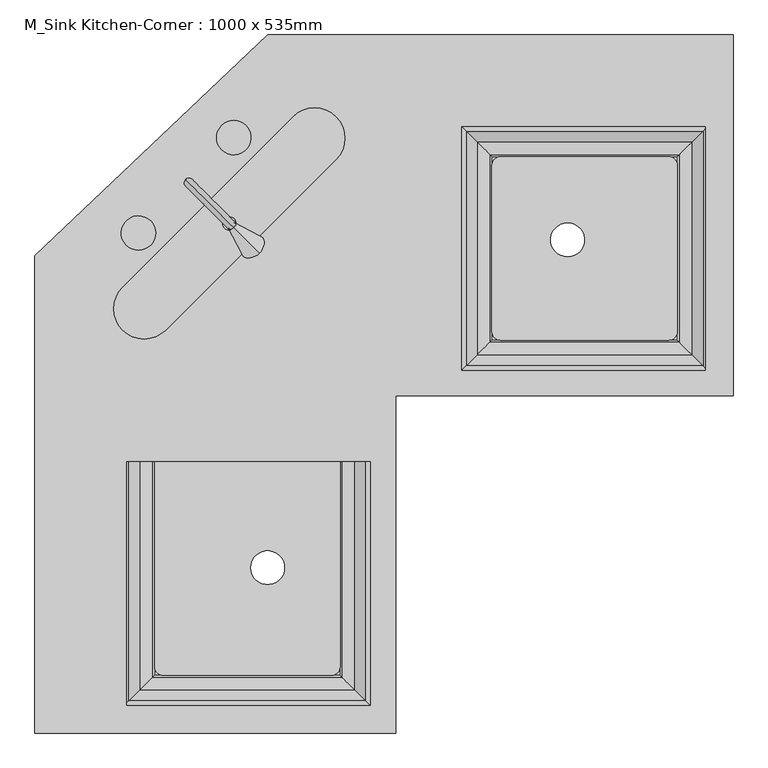
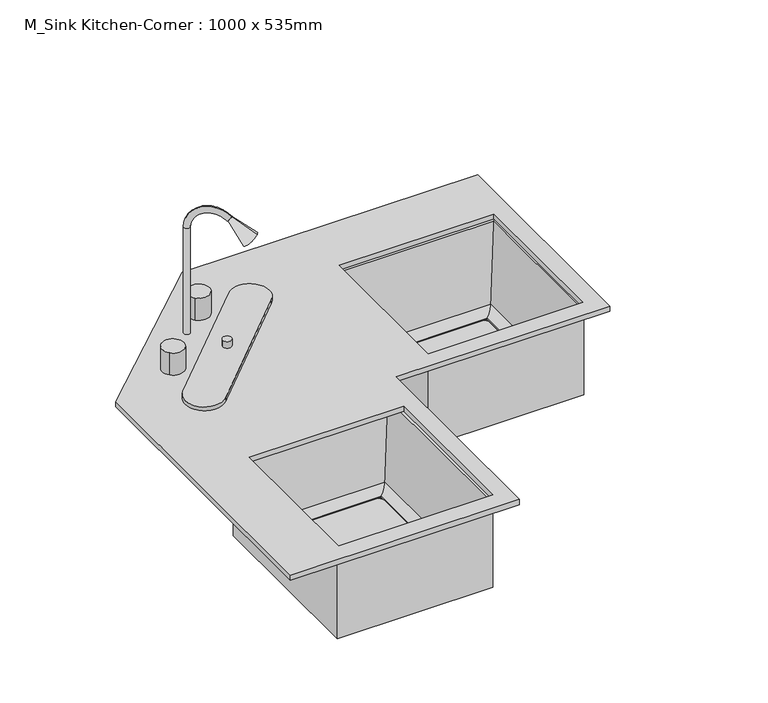
"""IFC4 building model written with IfcOpenShell, lengths in millimetres: flow terminal geometry, M_Sink Kitchen-Corner : 1000 x 535mm."""

from ifc_helpers import new_model, si_unit, point, frame, frame_2d, origin, place, context, project, spatial, polyline, circle_curve, ellipse_curve, trimmed, segment, composite_curve, outline, extrude, source, transform, mapped, element, save
from ifc_brep_helpers import plane_surface, cylinder_surface, revolved_surface, advanced_brep


def m_sink_kitchen_corner_1000_x_535mm_64178851(model_context):
    return source(origin(), model_context, "Body", "SolidModel", [
        extrude(outline(composite_curve([segment(trimmed(circle_curve(frame_2d((534.2861612, -1303.309682)), 12.7), [point((546.9861612, -1303.309682))], [point((534.2861612, -1316.009682))], False, "CARTESIAN"), True, "CONTINUOUS"), segment(polyline([(534.2861612, -1316.009682), (284.7743897, -1316.009682)]), True, "CONTINUOUS"), segment(trimmed(circle_curve(frame_2d((284.7743897, -1303.309682)), 12.7), [point((284.7743897, -1316.009682))], [point((272.0743897, -1303.309682))], False, "CARTESIAN"), True, "CONTINUOUS"), segment(polyline([(272.0743897, -1303.309682), (272.0743897, -1056.8979105)]), True, "CONTINUOUS"), segment(trimmed(circle_curve(frame_2d((284.7743897, -1056.8979105)), 12.7), [point((272.0743897, -1056.8979105))], [point((284.7743897, -1044.1979105))], False, "CARTESIAN"), True, "CONTINUOUS"), segment(polyline([(284.7743897, -1044.1979105), (534.2861612, -1044.1979105)]), True, "CONTINUOUS"), segment(trimmed(circle_curve(frame_2d((534.2861612, -1056.8979105)), 12.7), [point((534.2861612, -1044.1979105))], [point((546.9861612, -1056.8979105))], False, "CARTESIAN"), True, "CONTINUOUS"), segment(polyline([(546.9861612, -1056.8979105), (546.9861612, -1303.309682)]), True, "CONTINUOUS")], self_intersect=False), holes=[composite_curve([segment(trimmed(circle_curve(frame_2d((384.1861612, -1167.359682)), 25.0), [point((384.1861612, -1142.359682))], [point((384.1861612, -1192.359682))], True, "CARTESIAN"), True, "CONTINUOUS"), segment(trimmed(circle_curve(frame_2d((384.1861612, -1167.359682)), 25.0), [point((384.1861612, -1192.359682))], [point((384.1861612, -1142.359682))], True, "CARTESIAN"), True, "CONTINUOUS")], self_intersect=False)]), frame((0.0, 0.0, 684.1), z_axis=(0.0, 0.0, 1.0), x_axis=(1.0, 0.0, 0.0)), (0.0, 0.0, 1.0), 9.525),
        extrude(outline(composite_curve([segment(trimmed(circle_curve(frame_2d((34.2861612, -1493.809682)), 12.7), [point((34.2861612, -1481.109682))], [point((46.9861612, -1493.809682))], False, "CARTESIAN"), True, "CONTINUOUS"), segment(polyline([(46.9861612, -1493.809682), (46.9861612, -1800.209682)]), True, "CONTINUOUS"), segment(trimmed(circle_curve(frame_2d((34.2861612, -1800.209682)), 12.7), [point((46.9861612, -1800.209682))], [point((34.2861612, -1812.909682))], False, "CARTESIAN"), True, "CONTINUOUS"), segment(polyline([(34.2861612, -1812.909682), (-215.2256103, -1812.909682)]), True, "CONTINUOUS"), segment(trimmed(circle_curve(frame_2d((-215.2256103, -1800.209682)), 12.7), [point((-215.2256103, -1812.909682))], [point((-227.9256103, -1800.209682))], False, "CARTESIAN"), True, "CONTINUOUS"), segment(polyline([(-227.9256103, -1800.209682), (-227.9256103, -1493.809682)]), True, "CONTINUOUS"), segment(trimmed(circle_curve(frame_2d((-215.2256103, -1493.809682)), 12.7), [point((-227.9256103, -1493.809682))], [point((-215.2256103, -1481.109682))], False, "CARTESIAN"), True, "CONTINUOUS"), segment(polyline([(-215.2256103, -1481.109682), (34.2861612, -1481.109682)]), True, "CONTINUOUS")], self_intersect=False), holes=[composite_curve([segment(trimmed(circle_curve(frame_2d((-60.4756103, -1653.359682)), 25.0), [point((-85.4756103, -1653.359682))], [point((-35.4756103, -1653.359682))], True, "CARTESIAN"), True, "CONTINUOUS"), segment(trimmed(circle_curve(frame_2d((-60.4756103, -1653.359682)), 25.0), [point((-35.4756103, -1653.359682))], [point((-85.4756103, -1653.359682))], True, "CARTESIAN"), True, "CONTINUOUS")], self_intersect=False)]), frame((0.0, 0.0, 684.1), z_axis=(0.0, 0.0, 1.0), x_axis=(1.0, 0.0, 0.0)), (0.0, 0.0, 1.0), 9.525),
        advanced_brep(
        [(91.4361612, -1436.659682, 684.1), (91.4361612, -1436.659682, 900.0), (91.4361612, -1857.359682, 900.0), (91.4361612, -1857.359682, 684.1), (46.9861612, -1481.109682, 684.1), (46.9861612, -1812.909682, 684.1), (46.9861612, -1481.109682, 693.625), (46.9861612, -1812.909682, 693.625), (49.5745794, -1478.5212638, 693.625), (49.5745794, -1815.4981002, 693.625), (68.5520884, -1459.5437548, 711.0146831), (68.5520884, -1834.4756092, 711.0146831), (85.0861612, -1443.009682, 900.0), (85.0861612, -1851.009682, 900.0), (-272.3756103, -1857.359682, 900.0), (-272.3756103, -1857.359682, 684.1), (-227.9256103, -1812.909682, 684.1), (-227.9256103, -1812.909682, 693.625), (-230.5140285, -1815.4981002, 693.625), (-249.4915375, -1834.4756092, 711.0146831), (-266.0256103, -1851.009682, 900.0), (-272.3756103, -1436.659682, 900.0), (-272.3756103, -1436.659682, 684.1), (-227.9256103, -1481.109682, 684.1), (-227.9256103, -1481.109682, 693.625), (-230.5140285, -1478.5212638, 693.625), (-249.4915375, -1459.5437548, 711.0146831), (-266.0256103, -1443.009682, 900.0)],
        [
            (0, 1),
            (1, 2),
            (2, 3),
            (3, 0),
            (4, 0),
            (3, 5),
            (5, 4),
            (6, 4),
            (5, 7),
            (7, 6),
            (8, 6),
            (7, 9),
            (9, 8),
            (10, 8, ellipse_curve(frame((49.5745794, -1478.5212638, 712.675), z_axis=(-0.7071067811865475, 0.7071067811865475, 0.0), x_axis=(-0.7071067811865474, -0.7071067811865476, 0.0)), 26.9407684, 19.05)),
            (9, 11, ellipse_curve(frame((49.5745794, -1815.4981002, 712.675), z_axis=(-0.7071067811865475, -0.7071067811865475, 0.0), x_axis=(0.7071067811865474, -0.7071067811865476, 0.0)), 26.9407684, 19.05)),
            (11, 10),
            (12, 10),
            (11, 13),
            (13, 12),
            (1, 12),
            (13, 2),
            (2, 14),
            (14, 15),
            (15, 3),
            (15, 16),
            (16, 5),
            (16, 17),
            (17, 7),
            (17, 18),
            (18, 9),
            (18, 19, ellipse_curve(frame((-230.5140285, -1815.4981002, 712.675), z_axis=(-0.7071067811865475, 0.7071067811865475, 0.0), x_axis=(-0.7071067811865476, -0.7071067811865474, 0.0)), 26.9407684, 19.05)),
            (19, 11),
            (19, 20),
            (20, 13),
            (20, 14),
            (14, 21),
            (21, 22),
            (22, 15),
            (22, 23),
            (23, 16),
            (23, 24),
            (24, 17),
            (24, 25),
            (25, 18),
            (25, 26, ellipse_curve(frame((-230.5140285, -1478.5212638, 712.675), z_axis=(0.7071067811865475, 0.7071067811865475, 0.0), x_axis=(-0.7071067811865474, 0.7071067811865476, 0.0)), 26.9407684, 19.05)),
            (26, 19),
            (26, 27),
            (27, 20),
            (27, 21),
            (21, 1),
            (0, 22),
            (4, 23),
            (6, 24),
            (8, 25),
            (10, 26),
            (12, 27),
        ],
        [
            plane_surface(frame((91.4361612, -1436.659682, 900.0), z_axis=(1.0, 0.0, 0.0), x_axis=(0.0, -1.0, 0.0))),
            plane_surface(frame((91.4361612, -1436.659682, 684.1), z_axis=(0.0, 0.0, -1.0), x_axis=(0.0, -1.0, 0.0))),
            plane_surface(frame((46.9861612, -1481.109682, 684.1), z_axis=(-1.0, 0.0, 0.0), x_axis=(0.0, -1.0, 0.0))),
            plane_surface(frame((46.9861612, -1481.109682, 693.625), z_axis=(0.0, 0.0, 1.0), x_axis=(0.0, -1.0, 0.0))),
            revolved_surface(polyline([(68.6245794, -1834.5481002260162, 712.675), (68.6245794, -1459.4712637739838, 712.675)]), (49.5745794, -1436.659682, 712.675), (0.0, -1.0, 0.0)),
            plane_surface(frame((68.5520884, -1459.5437548, 711.0146831), z_axis=(-0.9961946980917438, 0.0, 0.08715574274767916), x_axis=(0.0, -1.0, 0.0))),
            plane_surface(frame((85.0861612, -1443.009682, 900.0), z_axis=(0.0, 0.0, 1.0), x_axis=(0.0, -1.0, 0.0))),
            plane_surface(frame((91.4361612, -1857.359682, 900.0), z_axis=(0.0, -1.0, 0.0), x_axis=(-1.0, 0.0, 0.0))),
            plane_surface(frame((91.4361612, -1857.359682, 684.1), z_axis=(0.0, 0.0, -1.0), x_axis=(-1.0, 0.0, 0.0))),
            plane_surface(frame((46.9861612, -1812.909682, 684.1), z_axis=(0.0, 1.0, 0.0), x_axis=(-1.0, 0.0, 0.0))),
            plane_surface(frame((46.9861612, -1812.909682, 693.625), z_axis=(0.0, 0.0, 1.0), x_axis=(-1.0, 0.0, 0.0))),
            revolved_surface(polyline([(-249.56402852601627, -1834.5481002, 712.675), (68.62457942601625, -1834.5481002, 712.675)]), (91.4361612, -1815.4981002, 712.675), (-1.0, 0.0, 0.0)),
            plane_surface(frame((68.5520884, -1834.4756092, 711.0146831), z_axis=(0.0, 0.9961946980917438, 0.08715574274767916), x_axis=(-1.0, 0.0, 0.0))),
            plane_surface(frame((85.0861612, -1851.009682, 900.0), z_axis=(0.0, 0.0, 1.0), x_axis=(-1.0, 0.0, 0.0))),
            plane_surface(frame((-272.3756103, -1857.359682, 900.0), z_axis=(-1.0, 0.0, 0.0), x_axis=(0.0, 1.0, 0.0))),
            plane_surface(frame((-272.3756103, -1857.359682, 684.1), z_axis=(0.0, 0.0, -1.0), x_axis=(0.0, 1.0, 0.0))),
            plane_surface(frame((-227.9256103, -1812.909682, 684.1), z_axis=(1.0, 0.0, 0.0), x_axis=(0.0, 1.0, 0.0))),
            plane_surface(frame((-227.9256103, -1812.909682, 693.625), z_axis=(0.0, 0.0, 1.0), x_axis=(0.0, 1.0, 0.0))),
            revolved_surface(polyline([(-249.5640285, -1459.4712637739838, 712.675), (-249.5640285, -1834.5481002260162, 712.675)]), (-230.5140285, -1857.359682, 712.675), (0.0, 1.0, 0.0)),
            plane_surface(frame((-249.4915375, -1834.4756092, 711.0146831), z_axis=(0.9961946980917438, 0.0, 0.08715574274767916), x_axis=(0.0, 1.0, 0.0))),
            plane_surface(frame((-266.0256103, -1851.009682, 900.0), z_axis=(0.0, 0.0, 1.0), x_axis=(0.0, 1.0, 0.0))),
            plane_surface(frame((-272.3756103, -1436.659682, 900.0), z_axis=(0.0, 1.0, 0.0), x_axis=(1.0, 0.0, 0.0))),
            plane_surface(frame((-272.3756103, -1436.659682, 684.1), z_axis=(0.0, 0.0, -1.0), x_axis=(1.0, 0.0, 0.0))),
            plane_surface(frame((-227.9256103, -1481.109682, 684.1), z_axis=(0.0, -1.0, 0.0), x_axis=(1.0, 0.0, 0.0))),
            plane_surface(frame((-227.9256103, -1481.109682, 693.625), z_axis=(0.0, 0.0, 1.0), x_axis=(1.0, 0.0, 0.0))),
            revolved_surface(polyline([(68.62457942601628, -1459.4712638, 712.675), (-249.56402852601624, -1459.4712638, 712.675)]), (-272.3756103, -1478.5212638, 712.675), (1.0, 0.0, 0.0)),
            plane_surface(frame((-249.4915375, -1459.5437548, 711.0146831), z_axis=(0.0, -0.9961946980917438, 0.08715574274767916), x_axis=(1.0, 0.0, 0.0))),
            plane_surface(frame((-266.0256103, -1443.009682, 900.0), z_axis=(0.0, 0.0, 1.0), x_axis=(1.0, 0.0, 0.0))),
        ],
        [
            (0, [[1, 2, 3, 4]]),
            (1, [[5, -4, 6, 7]]),
            (2, [[8, -7, 9, 10]]),
            (3, [[11, -10, 12, 13]]),
            (4, [[14, -13, 15, 16]]),
            (5, [[17, -16, 18, 19]]),
            (6, [[20, -19, 21, -2]]),
            (7, [[-3, 22, 23, 24]]),
            (8, [[-6, -24, 25, 26]]),
            (9, [[-9, -26, 27, 28]]),
            (10, [[-12, -28, 29, 30]]),
            (11, [[-15, -30, 31, 32]]),
            (12, [[-18, -32, 33, 34]]),
            (13, [[-21, -34, 35, -22]]),
            (14, [[-23, 36, 37, 38]]),
            (15, [[-25, -38, 39, 40]]),
            (16, [[-27, -40, 41, 42]]),
            (17, [[-29, -42, 43, 44]]),
            (18, [[-31, -44, 45, 46]]),
            (19, [[-33, -46, 47, 48]]),
            (20, [[-35, -48, 49, -36]]),
            (21, [[-37, 50, -1, 51]]),
            (22, [[-39, -51, -5, 52]]),
            (23, [[-41, -52, -8, 53]]),
            (24, [[-43, -53, -11, 54]]),
            (25, [[-45, -54, -14, 55]]),
            (26, [[-47, -55, -17, 56]]),
            (27, [[-49, -56, -20, -50]]),
        ],
    ),
        extrude(outline(composite_curve([segment(trimmed(circle_curve(frame_2d((-252.012502, -1157.1953436)), 25.4), [point((-269.9730143, -1175.1558558))], [point((-234.0519898, -1139.2348313))], False, "CARTESIAN"), True, "CONTINUOUS"), segment(trimmed(circle_curve(frame_2d((-252.012502, -1157.1953436)), 25.4), [point((-234.0519898, -1139.2348313))], [point((-269.9730143, -1175.1558558))], False, "CARTESIAN"), True, "CONTINUOUS")], self_intersect=False)), frame((0.0, 0.0, 921.7557241), z_axis=(0.0, 0.0, 1.0), x_axis=(1.0, 0.0, 0.0)), (0.0, 0.0, 1.0), 54.4442759),
        extrude(outline(composite_curve([segment(trimmed(circle_curve(frame_2d((-110.5911458, -1015.7739873)), 25.4), [point((-128.551658, -1033.7344996))], [point((-92.6306335, -997.8134751))], False, "CARTESIAN"), True, "CONTINUOUS"), segment(trimmed(circle_curve(frame_2d((-110.5911458, -1015.7739873)), 25.4), [point((-92.6306335, -997.8134751))], [point((-128.551658, -1033.7344996))], False, "CARTESIAN"), True, "CONTINUOUS")], self_intersect=False)), frame((0.0, 0.0, 921.7557241), z_axis=(0.0, 0.0, 1.0), x_axis=(1.0, 0.0, 0.0)), (0.0, 0.0, 1.0), 54.4442759),
        advanced_brep(
        [(591.4361612, -999.7479105, 684.1), (591.4361612, -999.7479105, 900.0), (591.4361612, -1360.459682, 900.0), (591.4361612, -1360.459682, 684.1), (546.9861612, -1044.1979105, 684.1), (546.9861612, -1316.009682, 684.1), (546.9861612, -1044.1979105, 693.625), (546.9861612, -1316.009682, 693.625), (549.5745794, -1041.6094923, 693.625), (549.5745794, -1318.5981002, 693.625), (568.5520884, -1022.6319833, 711.0146831), (568.5520884, -1337.5756092, 711.0146831), (585.0861612, -1006.0979105, 900.0), (585.0861612, -1354.109682, 900.0), (227.6243897, -1360.459682, 900.0), (227.6243897, -1360.459682, 684.1), (272.0743897, -1316.009682, 684.1), (272.0743897, -1316.009682, 693.625), (269.4859715, -1318.5981002, 693.625), (250.5084625, -1337.5756092, 711.0146831), (233.9743897, -1354.109682, 900.0), (227.6243897, -999.7479105, 900.0), (227.6243897, -999.7479105, 684.1), (272.0743897, -1044.1979105, 684.1), (272.0743897, -1044.1979105, 693.625), (269.4859715, -1041.6094923, 693.625), (250.5084625, -1022.6319833, 711.0146831), (233.9743897, -1006.0979105, 900.0)],
        [
            (0, 1),
            (1, 2),
            (2, 3),
            (3, 0),
            (4, 0),
            (3, 5),
            (5, 4),
            (6, 4),
            (5, 7),
            (7, 6),
            (8, 6),
            (7, 9),
            (9, 8),
            (10, 8, ellipse_curve(frame((549.5745794, -1041.6094923, 712.675), z_axis=(-0.7071067811865475, 0.7071067811865475, 0.0), x_axis=(-0.7071067811865474, -0.7071067811865476, 0.0)), 26.9407684, 19.05)),
            (9, 11, ellipse_curve(frame((549.5745794, -1318.5981002, 712.675), z_axis=(-0.7071067811865475, -0.7071067811865475, 0.0), x_axis=(0.7071067811865474, -0.7071067811865476, 0.0)), 26.9407684, 19.05)),
            (11, 10),
            (12, 10),
            (11, 13),
            (13, 12),
            (1, 12),
            (13, 2),
            (2, 14),
            (14, 15),
            (15, 3),
            (15, 16),
            (16, 5),
            (16, 17),
            (17, 7),
            (17, 18),
            (18, 9),
            (18, 19, ellipse_curve(frame((269.4859715, -1318.5981002, 712.675), z_axis=(-0.7071067811865475, 0.7071067811865475, 0.0), x_axis=(-0.7071067811865476, -0.7071067811865474, 0.0)), 26.9407684, 19.05)),
            (19, 11),
            (19, 20),
            (20, 13),
            (20, 14),
            (14, 21),
            (21, 22),
            (22, 15),
            (22, 23),
            (23, 16),
            (23, 24),
            (24, 17),
            (24, 25),
            (25, 18),
            (25, 26, ellipse_curve(frame((269.4859715, -1041.6094923, 712.675), z_axis=(0.7071067811865475, 0.7071067811865475, 0.0), x_axis=(-0.7071067811865474, 0.7071067811865476, 0.0)), 26.9407684, 19.05)),
            (26, 19),
            (26, 27),
            (27, 20),
            (27, 21),
            (21, 1),
            (0, 22),
            (4, 23),
            (6, 24),
            (8, 25),
            (10, 26),
            (12, 27),
        ],
        [
            plane_surface(frame((591.4361612, -999.7479105, 900.0), z_axis=(1.0, 0.0, 0.0), x_axis=(0.0, -1.0, 0.0))),
            plane_surface(frame((591.4361612, -999.7479105, 684.1), z_axis=(0.0, 0.0, -1.0), x_axis=(0.0, -1.0, 0.0))),
            plane_surface(frame((546.9861612, -1044.1979105, 684.1), z_axis=(-1.0, 0.0, 0.0), x_axis=(0.0, -1.0, 0.0))),
            plane_surface(frame((546.9861612, -1044.1979105, 693.625), z_axis=(0.0, 0.0, 1.0), x_axis=(0.0, -1.0, 0.0))),
            revolved_surface(polyline([(568.6245793999999, -1337.6481002260164, 712.675), (568.6245793999999, -1022.5594922739838, 712.675)]), (549.5745794, -999.7479105, 712.675), (0.0, -1.0, 0.0)),
            plane_surface(frame((568.5520884, -1022.6319833, 711.0146831), z_axis=(-0.9961946980917438, 0.0, 0.08715574274767911), x_axis=(0.0, -1.0, 0.0))),
            plane_surface(frame((585.0861612, -1006.0979105, 900.0), z_axis=(0.0, 0.0, 1.0), x_axis=(0.0, -1.0, 0.0))),
            plane_surface(frame((591.4361612, -1360.459682, 900.0), z_axis=(0.0, -1.0, 0.0), x_axis=(-1.0, 0.0, 0.0))),
            plane_surface(frame((591.4361612, -1360.459682, 684.1), z_axis=(0.0, 0.0, -1.0), x_axis=(-1.0, 0.0, 0.0))),
            plane_surface(frame((546.9861612, -1316.009682, 684.1), z_axis=(0.0, 1.0, 0.0), x_axis=(-1.0, 0.0, 0.0))),
            plane_surface(frame((546.9861612, -1316.009682, 693.625), z_axis=(0.0, 0.0, 1.0), x_axis=(-1.0, 0.0, 0.0))),
            revolved_surface(polyline([(250.43597147398373, -1337.6481002, 712.675), (568.6245794260162, -1337.6481002, 712.675)]), (591.4361612, -1318.5981002, 712.675), (-1.0, 0.0, 0.0)),
            plane_surface(frame((568.5520884, -1337.5756092, 711.0146831), z_axis=(0.0, 0.9961946980917438, 0.08715574274767911), x_axis=(-1.0, 0.0, 0.0))),
            plane_surface(frame((585.0861612, -1354.109682, 900.0), z_axis=(0.0, 0.0, 1.0), x_axis=(-1.0, 0.0, 0.0))),
            plane_surface(frame((227.6243897, -1360.459682, 900.0), z_axis=(-1.0, 0.0, 0.0), x_axis=(0.0, 1.0, 0.0))),
            plane_surface(frame((227.6243897, -1360.459682, 684.1), z_axis=(0.0, 0.0, -1.0), x_axis=(0.0, 1.0, 0.0))),
            plane_surface(frame((272.0743897, -1316.009682, 684.1), z_axis=(1.0, 0.0, 0.0), x_axis=(0.0, 1.0, 0.0))),
            plane_surface(frame((272.0743897, -1316.009682, 693.625), z_axis=(0.0, 0.0, 1.0), x_axis=(0.0, 1.0, 0.0))),
            revolved_surface(polyline([(250.4359715, -1022.5594922739838, 712.675), (250.4359715, -1337.6481002260164, 712.675)]), (269.4859715, -1360.459682, 712.675), (0.0, 1.0, 0.0)),
            plane_surface(frame((250.5084625, -1337.5756092, 711.0146831), z_axis=(0.9961946980917438, 0.0, 0.08715574274767911), x_axis=(0.0, 1.0, 0.0))),
            plane_surface(frame((233.9743897, -1354.109682, 900.0), z_axis=(0.0, 0.0, 1.0), x_axis=(0.0, 1.0, 0.0))),
            plane_surface(frame((227.6243897, -999.7479105, 900.0), z_axis=(0.0, 1.0, 0.0), x_axis=(1.0, 0.0, 0.0))),
            plane_surface(frame((227.6243897, -999.7479105, 684.1), z_axis=(0.0, 0.0, -1.0), x_axis=(1.0, 0.0, 0.0))),
            plane_surface(frame((272.0743897, -1044.1979105, 684.1), z_axis=(0.0, -1.0, 0.0), x_axis=(1.0, 0.0, 0.0))),
            plane_surface(frame((272.0743897, -1044.1979105, 693.625), z_axis=(0.0, 0.0, 1.0), x_axis=(1.0, 0.0, 0.0))),
            revolved_surface(polyline([(568.6245794260162, -1022.5594923000001, 712.675), (250.43597147398376, -1022.5594923000001, 712.675)]), (227.6243897, -1041.6094923, 712.675), (1.0, 0.0, 0.0)),
            plane_surface(frame((250.5084625, -1022.6319833, 711.0146831), z_axis=(0.0, -0.9961946980917438, 0.08715574274767911), x_axis=(1.0, 0.0, 0.0))),
            plane_surface(frame((233.9743897, -1006.0979105, 900.0), z_axis=(0.0, 0.0, 1.0), x_axis=(1.0, 0.0, 0.0))),
        ],
        [
            (0, [[1, 2, 3, 4]]),
            (1, [[5, -4, 6, 7]]),
            (2, [[8, -7, 9, 10]]),
            (3, [[11, -10, 12, 13]]),
            (4, [[14, -13, 15, 16]]),
            (5, [[17, -16, 18, 19]]),
            (6, [[20, -19, 21, -2]]),
            (7, [[-3, 22, 23, 24]]),
            (8, [[-6, -24, 25, 26]]),
            (9, [[-9, -26, 27, 28]]),
            (10, [[-12, -28, 29, 30]]),
            (11, [[-15, -30, 31, 32]]),
            (12, [[-18, -32, 33, 34]]),
            (13, [[-21, -34, 35, -22]]),
            (14, [[-23, 36, 37, 38]]),
            (15, [[-25, -38, 39, 40]]),
            (16, [[-27, -40, 41, 42]]),
            (17, [[-29, -42, 43, 44]]),
            (18, [[-31, -44, 45, 46]]),
            (19, [[-33, -46, 47, 48]]),
            (20, [[-35, -48, 49, -36]]),
            (21, [[-37, 50, -1, 51]]),
            (22, [[-39, -51, -5, 52]]),
            (23, [[-41, -52, -8, 53]]),
            (24, [[-43, -53, -11, 54]]),
            (25, [[-45, -54, -14, 55]]),
            (26, [[-47, -55, -17, 56]]),
            (27, [[-49, -56, -20, -50]]),
        ],
    ),
        advanced_brep(
        [(-92.5156055, -1167.5645399, 1179.2484831), (-72.8764192, -1187.2037262, 1207.0224867), (-110.5495322, -1149.5306132, 1240.9881656), (-116.5329673, -1143.547178, 1232.5263104), (-82.6960123, -1177.384133, 1193.1354849), (-112.8790057, -1147.2011396, 1235.8206835)],
        [
            (0, 1, circle_curve(frame((-82.6960123, -1177.384133, 1193.1354849), z_axis=(-0.49999999999999867, 0.5000000000000016, 0.7071067811865476), x_axis=(0.4999999999999987, -0.5000000000000012, 0.7071067811865476)), 19.6391863)),
            (1, 2),
            (2, 3, circle_curve(frame((-113.5412497, -1146.5388956, 1236.757238), z_axis=(0.49999999999999867, -0.5000000000000016, -0.7071067811865476), x_axis=(0.4999999999999987, -0.5000000000000012, 0.7071067811865476)), 5.9834352)),
            (3, 0),
            (1, 0, circle_curve(frame((-82.6960123, -1177.384133, 1193.1354849), z_axis=(-0.49999999999999867, 0.5000000000000016, 0.7071067811865476), x_axis=(0.4999999999999987, -0.5000000000000012, 0.7071067811865476)), 19.6391863)),
            (3, 2, circle_curve(frame((-113.5412497, -1146.5388956, 1236.757238), z_axis=(0.49999999999999867, -0.5000000000000016, -0.7071067811865476), x_axis=(0.4999999999999987, -0.5000000000000012, 0.7071067811865476)), 5.9834352)),
            (4, 1),
            (0, 4),
            (2, 5),
            (5, 3),
        ],
        [
            revolved_surface(polyline([(-110.5495322, -1149.5306132, 1240.9881656), (-72.8764192, -1187.2037262, 1207.0224867)]), (-113.3639618, -1146.7161835, 1236.5065151), (0.49999999999999856, -0.5000000000000014, -0.7071067811865475)),
            plane_surface(frame((-82.6960123, -1177.384133, 1193.1354849), z_axis=(0.49999999999999883, -0.5000000000000013, -0.7071067811865476), x_axis=(0.4999999999999987, -0.5000000000000012, 0.7071067811865476))),
            revolved_surface(polyline([(-112.8790057, -1147.2011396, 1235.8206835), (-110.5495322, -1149.5306132, 1240.9881656)]), (-113.3639618, -1146.7161835, 1236.5065151), (0.49999999999999856, -0.5000000000000014, -0.7071067811865475)),
        ],
        [
            (0, [[1, 2, 3, 4]]),
            (0, [[5, -4, 6, -2]]),
            (1, [[7, -1, 8]]),
            (1, [[-8, -5, -7]]),
            (2, [[-3, 9, 10]]),
            (2, [[-6, -10, -9]]),
        ],
    ),
        advanced_brep(
        [(-181.8879859, -1077.8855682, 938.1), (-171.9700025, -1087.8035515, 938.1), (-181.8879859, -1077.8855682, 1199.1505143), (-171.9700025, -1087.8035515, 1199.1505143), (-110.2122993, -1149.5612547, 1240.9881656), (-117.2429571, -1142.530597, 1231.095113)],
        [
            (0, 1, circle_curve(frame((-176.9289942, -1082.8445599, 938.1), z_axis=(0.0, 0.0, -1.0), x_axis=(0.7071067811865465, -0.7071067811865486, 0.0)), 7.0130733)),
            (1, 0, circle_curve(frame((-176.9289942, -1082.8445599, 938.1), z_axis=(0.0, 0.0, -1.0), x_axis=(0.7071067811865465, -0.7071067811865486, 0.0)), 7.0130733)),
            (0, 2),
            (2, 3, circle_curve(frame((-176.9289942, -1082.8445599, 1199.1505143), z_axis=(0.0, 0.0, -1.0), x_axis=(0.7071067811865465, -0.7071067811865486, 0.0)), 7.0130733)),
            (3, 1),
            (3, 2, circle_curve(frame((-176.9289942, -1082.8445599, 1199.1505143), z_axis=(0.0, 0.0, -1.0), x_axis=(0.7071067811865465, -0.7071067811865486, 0.0)), 7.0130733)),
            (4, 5, circle_curve(frame((-113.7276282, -1146.0459258, 1236.0416393), z_axis=(0.49874315442238853, -0.49874315442239, -0.7088797724816315), x_axis=(-0.5012536941677378, 0.5012536941677393, -0.7053293331248818)), 7.0130733)),
            (5, 4, circle_curve(frame((-113.7276282, -1146.0459258, 1236.0416393), z_axis=(0.49874315442238853, -0.49874315442239, -0.7088797724816315), x_axis=(-0.5012536941677378, 0.5012536941677393, -0.7053293331248818)), 7.0130733)),
            (5, 3, circle_curve(frame((-139.9449026, -1119.8286514, 1199.1505143), z_axis=(-0.7071067811865486, -0.7071067811865465, 0.0), x_axis=(-0.7071067811865465, 0.7071067811865486, 0.0)), 45.2903306)),
            (2, 4, circle_curve(frame((-139.9449026, -1119.8286514, 1199.1505143), z_axis=(0.7071067811865486, 0.7071067811865465, 0.0), x_axis=(-0.7071067811865465, 0.7071067811865486, 0.0)), 59.3164771)),
        ],
        [
            plane_surface(frame((-277.3407231, -1183.2562888, 938.1), z_axis=(0.0, 0.0, -1.0), x_axis=(0.7071067811865486, 0.7071067811865465, 0.0))),
            cylinder_surface(frame((-176.9289942, -1082.8445599, 938.1), z_axis=(0.0, 0.0, -1.0), x_axis=(0.7071067811865465, -0.7071067811865486, 0.0)), 7.0130733),
            plane_surface(frame((-214.1393571, -1246.4576547, 1236.0416393), z_axis=(0.4987431544223885, -0.49874315442239003, -0.7088797724816316), x_axis=(0.7071067811865486, 0.7071067811865465, 0.0))),
            revolved_surface(trimmed(ellipse_curve(frame((-176.9289942, -1082.8445599, 1199.1505143), z_axis=(0.0, 0.0, -1.0), x_axis=(0.7071067811865465, -0.7071067811865486, 0.0)), 7.0130733, 7.0130733), [point((-181.8879859, -1077.8855682, 1199.1505143))], [point((-171.9700025, -1087.8035515, 1199.1505143))], True, "CARTESIAN"), (-240.3566315, -1220.2403803, 1199.1505143), (0.7071067811865486, 0.7071067811865465, 0.0)),
            revolved_surface(trimmed(ellipse_curve(frame((-176.9289942, -1082.8445599, 1199.1505143), z_axis=(0.0, 0.0, -1.0), x_axis=(0.7071067811865465, -0.7071067811865486, 0.0)), 7.0130733, 7.0130733), [point((-171.9700025, -1087.8035515, 1199.1505143))], [point((-181.8879859, -1077.8855682, 1199.1505143))], True, "CARTESIAN"), (-240.3566315, -1220.2403803, 1199.1505143), (0.7071067811865486, 0.7071067811865465, 0.0)),
        ],
        [
            (0, [[1, 2]]),
            (1, [[-1, 3, 4, 5]]),
            (1, [[-2, -5, 6, -3]]),
            (2, [[7, 8]]),
            (3, [[9, -4, 10, -8]]),
            (4, [[-10, -6, -9, -7]]),
        ],
    ),
        extrude(outline(composite_curve([segment(trimmed(circle_curve(frame_2d((-117.2742684, -1142.9992524)), 10.0), [point((-127.2742684, -1142.9992524))], [point((-107.2742684, -1142.9992524))], False, "CARTESIAN"), True, "CONTINUOUS"), segment(trimmed(circle_curve(frame_2d((-117.2742684, -1142.9992524)), 10.0), [point((-107.2742684, -1142.9992524))], [point((-127.2742684, -1142.9992524))], False, "CARTESIAN"), True, "CONTINUOUS")], self_intersect=False)), frame((0.0, 0.0, 921.7557241), z_axis=(0.0, 0.0, 1.0), x_axis=(1.0, 0.0, 0.0)), (0.0, 0.0, 1.0), 16.3442759),
        extrude(outline(composite_curve([segment(trimmed(circle_curve(frame_2d((9.1006766, -1016.6243074)), 45.0), [point((-22.7191286, -984.8045022))], [point((40.9204817, -1048.4441125))], False, "CARTESIAN"), True, "CONTINUOUS"), segment(polyline([(40.9204817, -1048.4441125), (-211.8294083, -1301.1940025)]), True, "CONTINUOUS"), segment(trimmed(circle_curve(frame_2d((-243.6492134, -1269.3741974)), 45.0), [point((-211.8294083, -1301.1940025))], [point((-275.4690186, -1237.5543922))], False, "CARTESIAN"), True, "CONTINUOUS"), segment(polyline([(-275.4690186, -1237.5543922), (-22.7191286, -984.8045022)]), True, "CONTINUOUS")], self_intersect=False)), frame((0.0, 0.0, 912.7), z_axis=(0.0, 0.0, 1.0), x_axis=(1.0, 0.0, 0.0)), (0.0, 0.0, 1.0), 9.0557241),
        extrude(outline(polyline([(629.5361612, -1398.559682), (129.5361612, -1398.559682), (129.5361612, -1898.559682), (-405.4638388, -1898.559682), (-405.4638388, -1191.0479105), (-60.4756103, -863.559682), (629.5361612, -863.559682), (629.5361612, -1398.559682)]), holes=[polyline([(588.3361612, -1360.459682), (588.3361612, -999.7479105), (227.6243897, -999.7479105), (227.6243897, -1360.459682), (588.3361612, -1360.459682)]), polyline([(-269.2756103, -1857.359682), (91.4361612, -1857.359682), (91.4361612, -1496.6479105), (-269.2756103, -1496.6479105), (-269.2756103, -1857.359682)])]), frame((0.0, 0.0, 900.0), z_axis=(0.0, 0.0, 1.0), x_axis=(1.0, 0.0, 0.0)), (0.0, 0.0, 1.0), 12.7),
    ])


if __name__ == "__main__":
    model = new_model("IFC4")
    model_context = context("Model", 3, world=origin())
    ifc_project = project(units=[si_unit("LENGTHUNIT", "METRE", prefix="MILLI")], contexts=[model_context])
    site = spatial("IfcSite", under=ifc_project)
    building = spatial("IfcBuilding", under=site)
    placement = place(None, origin())
    m_sink_kitchen_corner_1000_x_535mm_shape = m_sink_kitchen_corner_1000_x_535mm_64178851(model_context)
    element("IfcFlowTerminal", 1, ObjectType="M_Sink Kitchen-Corner : 1000 x 535mm", at=placement, inside=building, context=model_context, shape_type="MappedRepresentation", body=[
        mapped(m_sink_kitchen_corner_1000_x_535mm_shape, transform((0.0, 0.0, 0.0), x_axis=(1.0, 0.0, 0.0), y_axis=(0.0, 1.0, 0.0), z_axis=(0.0, 0.0, 1.0))),
    ])
    save(model, "model.ifc")

# Revit data of these elements
# Type "M_Sink Kitchen-Corner : 1000 x 535mm"
#   Sink Offset (Side) [instance default] = 0' - 1.62205"
#   Sink Offset (Front) = 0' - 1 1/2"
#   Sink Length [instance default] = 1' - 4.56299"
#   Counter Height [instance default] = 2' - 11.43307"
#   Depth = 1' - 9.06299"
#   Width = 1' - 9.06299"
#   Fixture Material = Metal - Steel, Polished
#   Sink Material = Metal - Steel, Polished
#   Default Elevation = 0
#   Assembly Code = ""
# Element 1 (IfcFlowTerminal, "M_Sink Kitchen-Corner : 1000 x 535mm")
#   Sink Length = 1' - 2.20125"
#   Materials on its faces: "Metal - Steel, Polished"
# Materials
#   "Metal - Steel, Polished": colour RGB 192 192 192, transparency 0
